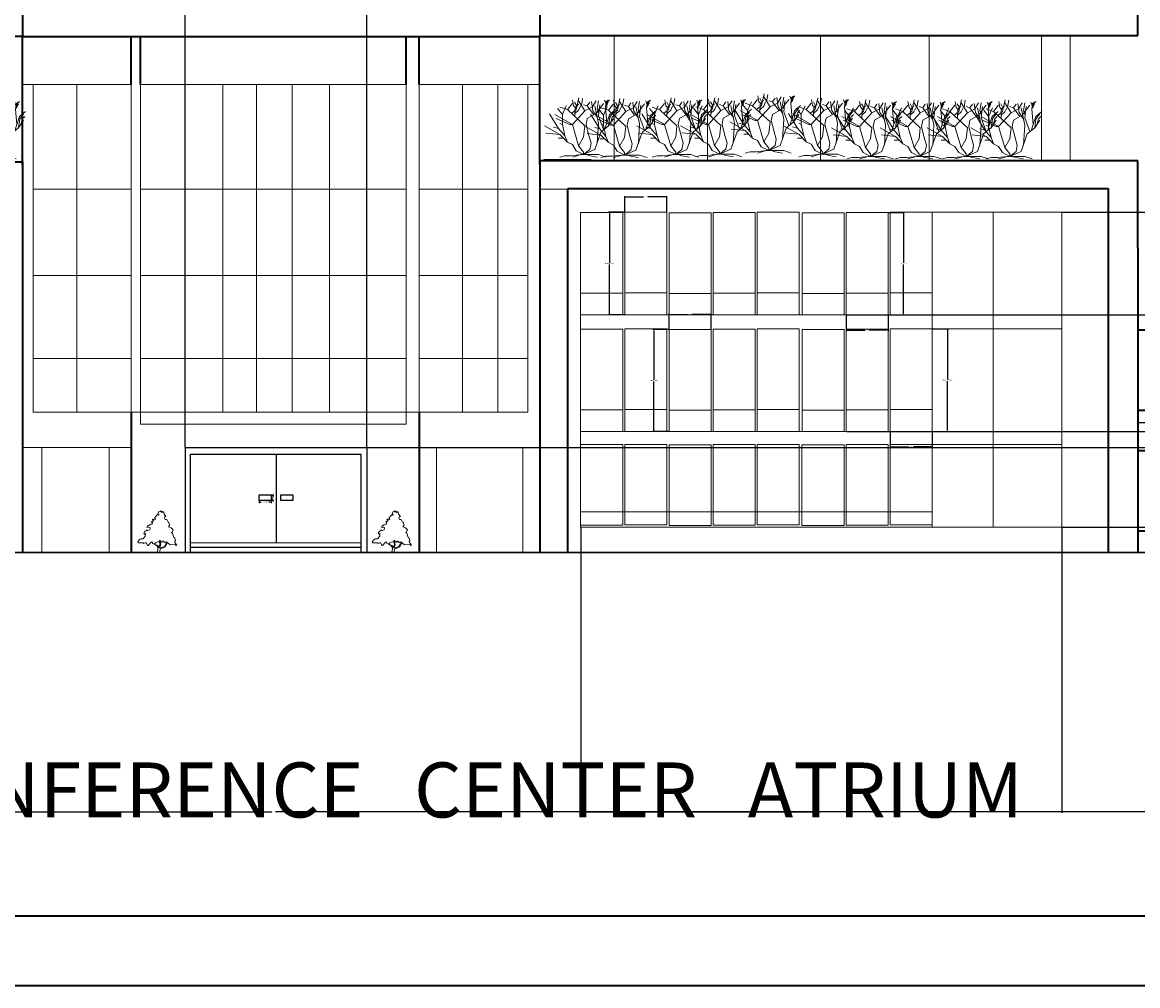
# Model space of a CAD drawing. Units: inches. Extents: x -279 to 364, y -385 to 335.
# Tile 2 of 9: x 7 to 238, y -385 to -185. Entities that reach past the tile are written whole.
import ezdxf

# ---------------------------------------------------------------- set-up
doc = ezdxf.new("R2010")
doc.units = ezdxf.units.IN
doc.header["$MEASUREMENT"] = 0
for name, color, linetype, lineweight in [('A-ANNO-DIMS', 2, 'Continuous', 18), ('A-ANNO-TEXT', 7, 'Continuous', 25), ('A-ANNO-TTLB', 7, 'Continuous', 35), ('A-DOOR', 3, 'Continuous', 25), ('A-GLAZ', 4, 'Continuous', 18), ('A-GLAZ-CURT', 4, 'Continuous', 18), ('A-WALL', 7, 'Continuous', 35), ('C-TOPO', 32, 'Continuous', 30), ('L-PLNT', 94, 'Continuous', 13)]:
    doc.layers.add(name, color=color, linetype=linetype, lineweight=lineweight)
doc.styles.get("Standard").update_dxf_attribs({"font": 'arial.ttf'})
doc.dimstyles.get("Standard").update_dxf_attribs({"dimtxt": 0.18, "dimasz": 0.18, "dimexe": 0.18, "dimexo": 0.0625, "dimgap": 0.09, "dimtad": 0, "dimtih": 1, "dimtoh": 1, "dimdec": 4, "dimzin": 0, "dimdsep": 46, "dimtxsty": 'Standard', "dimcen": 0.09, "dimadec": 0, "dimazin": 0, "dimtfac": 1, "dimtdec": 4, "dimtofl": 0, "dimtmove": 0, "dimatfit": 3, "dimfxl": 1, "dimtolj": 1, "dimtzin": 0, "dimarcsym": 0})

# ---------------------------------------------------------------- blocks, each defined once
blk = doc.blocks.new('*U2')
for p, q in [((-12.471, 19.775), (-12.898, 22.044)), ((-11.433, 18.289), (-10.457, 22.749)), ((-8.16, 17.76), (-10.56, 21.6)), ((-9.48, 19.775), (-8.992, 22.592)), ((-5.28, 19.2), (-3.84, 21.6)), ((-3.377, 18.602), (-2.888, 21.575)), ((-0.508, 21.888), (-0.081, 20.558)), ((0.041, 20.714), (1.384, 22.044)), ((0.102, 21.34), (0.835, 21.888)), ((-16.8, 16.32), (-18.72, 18.72)), ((-14.88, 18.24), (-17.76, 19.2)), ((-16.8, 16.32), (-15.36, 19.68)), ((-14.88, 18.24), (-12.96, 20.64)), ((-8.16, 12), (-14.88, 18.24)), ((-13.325, 16.724), (-11.433, 18.289)), ((-12.96, 12.48), (-8.16, 17.76)), ((-11.677, 19.071), (-12.471, 19.775)), ((-11.28, 19.619), (-12.104, 21.184)), ((-12.043, 15.628), (-11.921, 18.836)), ((-11.982, 16.802), (-10.579, 18.054)), ((-11.921, 18.836), (-10.64, 20.401)), ((-10.579, 18.054), (-9.846, 19.697)), ((-7.2, 19.68), (-8.64, 20.16)), ((-8.16, 17.76), (-5.28, 19.2)), ((-7.2, 19.68), (-6.24, 21.12)), ((-4.8, 16.32), (-7.2, 19.68)), ((-5.086, 17.741), (-5.513, 21.34)), ((-3.377, 15.315), (-5.086, 17.819)), ((-2.88, 12.96), (-4.32, 19.68)), ((-3.84, 16.8), (-0.96, 20.64)), ((-2.766, 16.802), (-3.377, 18.602)), ((-2.88, 15.84), (-2.4, 20.16)), ((-0.203, 19.149), (0.102, 21.34)), ((0.346, 13.203), (-0.203, 19.149)), ((-0.142, 19.384), (0.59, 20.401)), ((-0.02, 20.01), (0.896, 21.105)), ((1.323, 16.254), (3.642, 18.289)), ((1.44, 15.36), (2.88, 17.28)), ((-18.24, 11.04), (-21.755, 16.655)), ((-12.96, 12.48), (-19.68, 16.32)), ((-13.92, 12.48), (-19.2, 14.88)), ((-16.8, 12.48), (-17.76, 12.96)), ((-16.8, 12.48), (-16.8, 16.32)), ((-7.68, 12.48), (-7.2, 14.88)), ((-7.2, 14.88), (-3.84, 16.8)), ((-3.36, 5.28), (-2.88, 12.96)), ((-0.96, 10.56), (-2.88, 15.84)), ((-0.48, 10.8), (0.346, 13.203)), ((0.346, 13.203), (1.323, 16.254)), ((0.96, 12), (1.44, 15.36)), ((0.96, 12), (2.88, 14.88)), ((1.92, 13.44), (2.4, 15.36)), ((2.4, 15.36), (3.36, 16.32)), ((-17.76, 8.64), (-23.663, 11.961)), ((-17.76, 8.64), (-23.128, 9.222)), ((-18.24, 11.04), (-20.16, 11.52)), ((-15.84, 8.16), (-18.24, 11.04)), ((-14.88, 5.76), (-17.76, 8.64)), ((-15.84, 8.16), (-16.8, 12.48)), ((-12.96, 12.48), (-13.92, 12.48)), ((-10.56, 4.32), (-12.96, 12.48)), ((-8.64, 7.68), (-8.16, 12)), ((-6.72, 8.64), (-7.68, 12.48)), ((-5.76, 5.28), (-6.72, 8.64)), ((-4.32, 2.88), (-1.92, 9.6)), ((-1.92, 9.6), (0.96, 12)), ((-16.32, 7.2), (-18.24, 7.2)), ((-14.88, 5.76), (-15.84, 8.16)), ((-12.96, 4.8), (-14.88, 5.76)), ((-11.52, 2.4), (-12.96, 4.8)), ((-10.56, 4.32), (-8.64, 7.68)), ((-8.64, 1.92), (-10.56, 4.32)), ((-6.24, 2.88), (-5.76, 5.28)), ((-15.84, 0.48), (-17.76, 0)), ((-13.44, 0.48), (-15.84, 0.48)), ((-9.6, 0.96), (-13.44, 0.48)), ((-9.6, 0.96), (-12.96, 0)), ((-8.64, 0.96), (-11.52, 2.4)), ((-9.6, 0.96), (-7.68, 0.96)), ((-8.64, 0.96), (-4.32, 2.88)), ((-8.64, 0.96), (-6.24, 2.88)), ((-8.64, 0.96), (-8.64, 1.92)), ((-8.64, 0.96), (-2.88, 0.96)), ((-7.68, 0.96), (-6.24, 0.48)), ((-6.24, 0.48), (-3.36, 0)), ((-2.88, 0.96), (0, 0))]:
    blk.add_line(p, q)
blk = doc.blocks.new('*U4')
for points in [[(22.0124, 137.721), (18.5475, 141.5624), (15.5282, 138.2446), (13.8028, 139.3505), (13.3714, 142.1153), (11.2148, 143.2214), (8.1954, 140.4564), (4.7447, 141.0094), (2.1567, 136.0326), (2.1567, 131.6088), (5.6074, 129.9499), (3.0193, 128.2909), (0.4313, 130.5029), (-6.9015, 123.3141), (-6.9015, 121.6552), (-9.9208, 119.9963), (-9.0581, 118.3373), (-6.9015, 115.0195), (-10.7835, 112.2546), (-14.6656, 115.0195), (-16.8222, 114.4665), (-17.6849, 112.2546), (-14.6656, 111.7016), (-14.2342, 107.2778), (-17.6065, 107.8307), (-21.5669, 103.9599), (-17.2536, 103.4069), (-18.9789, 97.8771), (-22.8609, 97.3241), (-27.1743, 94.5593), (-32.3504, 91.7944), (-32.7817, 94.0063), (-36.6638, 85.7116), (-29.7624, 87.3705), (-25.449, 84.6056), (-26.743, 77.9699), (-34.507, 75.205), (-37.9578, 77.4169), (-39.2518, 74.099), (-42.2711, 73.5461), (-44.8592, 70.2282), (-47.8786, 66.3574), (-43.9965, 63.0395), (-41.4085, 64.6985), (-44.3346, 59.8898), (-42.2089, 60.1377), (-42.5159, 55.7849), (-49.6039, 46.4502), (-58.2307, 45.8972), (-62.1127, 43.6853), (-68.5828, 36.4966), (-65.9947, 32.0727), (-50.0352, 32.6257), (-47.0159, 30.4138), (-39.6831, 33.7317), (-34.507, 22.6721), (-32.3504, 22.6721), (-22.4296, 34.8376), (-19.4102, 36.4966), (-17.2536, 33.7317), (-17.2536, 29.8608), (-13.8028, 28.7549), (-9.0581, 28.7549), (-7.3328, 32.6257), (-1.7254, 35.3906), (3.8821, 35.9436), (6.4701, 38.1555), (6.9014, 38.7085), (8.1954, 41.4734), (9.9208, 40.3674), (11.2148, 35.9436), (14.2341, 37.6025), (15.0968, 36.4966), (15.9595, 33.7317), (18.9789, 38.7085), (21.9982, 38.7085), (23.2922, 36.4966), (21.9982, 34.2847), (25.4489, 35.3906), (26.743, 33.7317), (29.7623, 35.9436), (32.7817, 34.8376), (38.8204, 28.7549), (41.4084, 27.6489), (43.5651, 25.437), (61.6813, 27.0959), (65.132, 23.7781), (67.7201, 24.884), (60.8186, 33.7317), (60.3873, 37.0495), (62.544, 40.3674), (58.662, 50.874), (56.5053, 50.874), (52.1919, 66.3574), (47.8785, 66.9103), (50.4665, 69.1222), (53.9172, 77.9699), (47.0158, 85.1586), (38.3891, 87.9235), (42.2711, 94.0063)], [(42.2711, 94.0063), (38.8204, 104.5129), (36.6637, 104.5129), (32.3503, 113.9135), (29.7623, 113.3605), (26.743, 113.3605), (24.5862, 117.7844), (25.8802, 123.8671), (29.331, 123.8671), (22.8609, 131.6088), (21.9982, 137.6916)], [(8.1954, 40.3674), (11.2148, 27.6489), (8.1954, 13.8245), (24.5862, 19.9072), (32.7817, 34.2847)], [(-12.9401, 28.7549), (-2.588, 22.1191), (0.8626, 17.6953), (1.7253, 11.6125), (0, 0)], [(-9.9208, 28.2019), (0, 23.2251), (3.4507, 19.9072), (4.7447, 15.4834), (8.6267, 27.0959), (6.4701, 37.6025)], [(34.5071, 33.1787), (27.1743, 18.2483), (9.0581, 10.5066), (7.7641, 3.8708), (8.1954, 0)]]:
    blk.add_lwpolyline(points)
blk = doc.blocks.new('WIN-SIDE-SINGLE')
for p, q in [((8.72, 16.72), (0, 16.72)), ((0, 16.72), (0, 15.47)), ((8.72, 0), (8.72, 16.72)), ((0, 15.47), (0, 0)), ((0, 0), (8.72, 0))]:
    blk.add_line(p, q)
blk = doc.blocks.new('WIN-ATRIUM-BAND')
for p, q in [((0, 0), (0, 21.21)), ((0, 21.21), (8.71, 21.21)), ((8.71, 21.21), (8.71, 19.97)), ((8.71, 19.97), (8.71, 0)), ((8.71, 4.5), (0, 4.5))]:
    blk.add_line(p, q)
blk = doc.blocks.new('WIN-ATRIUM-BAND-2')
for p, q in [((0, 0), (0, 21.26)), ((0, 21.26), (8.71, 21.26)), ((8.71, 21.26), (8.71, 20.01)), ((8.71, 20.01), (8.71, 0)), ((8.71, 4.54), (0, 4.54))]:
    blk.add_line(p, q)
blk = doc.blocks.new('WIN-ATRIUM-BAND-3')
for p, q in [((0, 0), (0, 21.12)), ((0, 21.12), (8.71, 21.12)), ((8.71, 21.12), (8.71, 19.88)), ((8.71, 19.88), (8.71, 0)), ((8.71, 4.4), (0, 4.4))]:
    blk.add_line(p, q)
blk = doc.blocks.new('PROJECTION-SIDE')
for p, q in [((0, 16.72), (5.49, 16.72)), ((5.49, 16.72), (5.49, 0)), ((5.49, 0), (0, 0))]:
    blk.add_line(p, q)
blk = doc.blocks.new('PULL-ATRIUM')
for p, q in [((0, 1.18), (2.49, 1.18)), ((0, 0), (0, 1.18)), ((2.49, 1.18), (2.49, 0)), ((2.49, 0), (0, 0))]:
    blk.add_line(p, q)
blk = doc.blocks.new('WIN-RIBBON-END')
for p, q in [((0, 0), (0, 21.26)), ((0, 21.26), (8.72, 21.26)), ((8.72, 21.26), (8.72, 20.01)), ((8.72, 20.01), (8.72, 4.54)), ((8.72, 4.54), (0, 4.54))]:
    blk.add_line(p, q)
blk = doc.blocks.new('*D52')
at = {"layer": 'A-ANNO-DIMS', "color": 0, "lineweight": -2, "transparency": 16777216}
for p, q in [((186.63, -224.9), (189.93, -224.9)), ((189.75, -225.08), (189.75, -235.32)), ((189.75, -245.93), (189.75, -235.69)), ((186.63, -246.11), (189.93, -246.11))]:
    blk.add_line(p, q, dxfattribs=at)
at = {"layer": 'A-ANNO-DIMS', "color": 0, "transparency": 16777216}
for points in [[(189.72, -225.08), (189.78, -225.08), (189.75, -224.9)], [(189.72, -245.93), (189.78, -245.93), (189.75, -246.11)]]:
    blk.add_solid(points, dxfattribs=at)
at = {"layer": 'Defpoints', "color": 0, "transparency": 16777216}
for p in [(186.57, -224.9), (189.75, -224.9), (186.57, -246.11)]:
    blk.add_point(p, dxfattribs=at)
at = {"layer": 'A-ANNO-DIMS', "color": 0, "transparency": 16777216, "insert": (189.75, -235.51), "char_height": 0.18, "attachment_point": 5}
blk.add_mtext('\\A1;LIGHT A 21 TYP.', dxfattribs=at)
blk = doc.blocks.new('*D53')
at = {"layer": 'A-ANNO-DIMS', "color": 0, "lineweight": -2, "transparency": 16777216}
for p, q in [((177.85, -246.17), (177.85, -249.47)), ((186.57, -246.17), (186.57, -249.47)), ((178.03, -249.29), (181.75, -249.29)), ((186.39, -249.29), (182.67, -249.29))]:
    blk.add_line(p, q, dxfattribs=at)
at = {"layer": 'A-ANNO-DIMS', "color": 0, "transparency": 16777216}
for points in [[(178.03, -249.26), (178.03, -249.32), (177.85, -249.29)], [(186.39, -249.26), (186.39, -249.32), (186.57, -249.29)]]:
    blk.add_solid(points, dxfattribs=at)
at = {"layer": 'Defpoints', "color": 0, "transparency": 16777216}
for p in [(177.85, -246.11), (186.57, -246.11), (186.57, -249.29)]:
    blk.add_point(p, dxfattribs=at)
at = {"layer": 'A-ANNO-DIMS', "color": 0, "transparency": 16777216, "insert": (182.21, -249.29), "char_height": 0.18, "attachment_point": 5}
blk.add_mtext('\\A1;9 TYP.', dxfattribs=at)
blk = doc.blocks.new('*D54')
at = {"layer": 'A-ANNO-DIMS', "color": 0, "lineweight": -2, "transparency": 16777216}
for p, q in [((131.88, -224.85), (128.57, -224.85)), ((128.75, -225.03), (128.75, -235.3)), ((128.75, -245.93), (128.75, -235.67)), ((131.88, -246.11), (128.57, -246.11))]:
    blk.add_line(p, q, dxfattribs=at)
at = {"layer": 'A-ANNO-DIMS', "color": 0, "transparency": 16777216}
for points in [[(128.72, -225.03), (128.78, -225.03), (128.75, -224.85)], [(128.72, -245.93), (128.78, -245.93), (128.75, -246.11)]]:
    blk.add_solid(points, dxfattribs=at)
at = {"layer": 'Defpoints', "color": 0, "transparency": 16777216}
for p in [(128.75, -224.85), (131.94, -224.85), (131.94, -246.11)]:
    blk.add_point(p, dxfattribs=at)
at = {"layer": 'A-ANNO-DIMS', "color": 0, "transparency": 16777216, "insert": (128.75, -235.48), "char_height": 0.18, "attachment_point": 5}
blk.add_mtext('\\A1;LIGHT B 21 TYP.', dxfattribs=at)
blk = doc.blocks.new('*D55')
at = {"layer": 'A-ANNO-DIMS', "color": 0, "lineweight": -2, "transparency": 16777216}
for p, q in [((131.94, -224.79), (131.94, -221.49)), ((132.12, -221.67), (135.84, -221.67)), ((140.47, -221.67), (136.75, -221.67)), ((140.65, -224.79), (140.65, -221.49))]:
    blk.add_line(p, q, dxfattribs=at)
at = {"layer": 'A-ANNO-DIMS', "color": 0, "transparency": 16777216}
for points in [[(132.12, -221.64), (132.12, -221.7), (131.94, -221.67)], [(140.47, -221.64), (140.47, -221.7), (140.65, -221.67)]]:
    blk.add_solid(points, dxfattribs=at)
at = {"layer": 'Defpoints', "color": 0, "transparency": 16777216}
for p in [(140.65, -221.67), (131.94, -224.85), (140.65, -224.85)]:
    blk.add_point(p, dxfattribs=at)
at = {"layer": 'A-ANNO-DIMS', "color": 0, "transparency": 16777216, "insert": (136.3, -221.67), "char_height": 0.18, "attachment_point": 5}
blk.add_mtext('\\A1;9 TYP.', dxfattribs=at)
blk = doc.blocks.new('*D56')
at = {"layer": 'A-ANNO-DIMS', "color": 0, "lineweight": -2, "transparency": 16777216}
for p, q in [((141.08, -249.18), (137.8, -249.18)), ((137.98, -249.36), (137.98, -259.56)), ((137.98, -270.13), (137.98, -259.93)), ((141.08, -270.31), (137.8, -270.31))]:
    blk.add_line(p, q, dxfattribs=at)
at = {"layer": 'A-ANNO-DIMS', "color": 0, "transparency": 16777216}
for points in [[(137.95, -249.36), (138.01, -249.36), (137.98, -249.18)], [(137.95, -270.13), (138.01, -270.13), (137.98, -270.31)]]:
    blk.add_solid(points, dxfattribs=at)
at = {"layer": 'Defpoints', "color": 0, "transparency": 16777216}
for p in [(137.98, -249.18), (141.15, -249.18), (141.15, -270.31)]:
    blk.add_point(p, dxfattribs=at)
at = {"layer": 'A-ANNO-DIMS', "color": 0, "transparency": 16777216, "insert": (137.98, -259.74), "char_height": 0.18, "attachment_point": 5}
blk.add_mtext('\\A1;LIGHT C 21 TYP.', dxfattribs=at)
blk = doc.blocks.new('*D57')
at = {"layer": 'A-ANNO-DIMS', "color": 0, "lineweight": -2, "transparency": 16777216}
for p, q in [((141.15, -249.12), (141.15, -245.83)), ((141.33, -246.01), (145.05, -246.01)), ((149.68, -246.01), (145.96, -246.01)), ((149.86, -249.12), (149.86, -245.83))]:
    blk.add_line(p, q, dxfattribs=at)
at = {"layer": 'A-ANNO-DIMS', "color": 0, "transparency": 16777216}
for points in [[(141.33, -245.98), (141.33, -246.04), (141.15, -246.01)], [(149.68, -245.98), (149.68, -246.04), (149.86, -246.01)]]:
    blk.add_solid(points, dxfattribs=at)
at = {"layer": 'Defpoints', "color": 0, "transparency": 16777216}
for p in [(149.86, -246.01), (141.15, -249.18), (149.86, -249.18)]:
    blk.add_point(p, dxfattribs=at)
at = {"layer": 'A-ANNO-DIMS', "color": 0, "transparency": 16777216, "insert": (145.5, -246.01), "char_height": 0.18, "attachment_point": 5}
blk.add_mtext('\\A1;9 TYP.', dxfattribs=at)
blk = doc.blocks.new('*D58')
at = {"layer": 'A-ANNO-DIMS', "color": 0, "lineweight": -2, "transparency": 16777216}
for p, q in [((195.77, -249.05), (199.08, -249.05)), ((198.9, -249.23), (198.9, -259.5)), ((198.9, -270.13), (198.9, -259.86)), ((195.77, -270.31), (199.08, -270.31))]:
    blk.add_line(p, q, dxfattribs=at)
at = {"layer": 'A-ANNO-DIMS', "color": 0, "transparency": 16777216}
for points in [[(198.87, -249.23), (198.93, -249.23), (198.9, -249.05)], [(198.87, -270.13), (198.93, -270.13), (198.9, -270.31)]]:
    blk.add_solid(points, dxfattribs=at)
at = {"layer": 'Defpoints', "color": 0, "transparency": 16777216}
for p in [(195.71, -249.05), (198.9, -249.05), (195.71, -270.31)]:
    blk.add_point(p, dxfattribs=at)
at = {"layer": 'A-ANNO-DIMS', "color": 0, "transparency": 16777216, "insert": (198.9, -259.68), "char_height": 0.18, "attachment_point": 5}
blk.add_mtext('\\A1;END PANEL 21 TYP.', dxfattribs=at)
blk = doc.blocks.new('*D59')
at = {"layer": 'A-ANNO-DIMS', "color": 0, "lineweight": -2, "transparency": 16777216}
for p, q in [((186.99, -270.37), (186.99, -273.67)), ((195.71, -270.37), (195.71, -273.67)), ((187.17, -273.49), (190.89, -273.49)), ((195.53, -273.49), (191.81, -273.49))]:
    blk.add_line(p, q, dxfattribs=at)
at = {"layer": 'A-ANNO-DIMS', "color": 0, "transparency": 16777216}
for points in [[(187.17, -273.46), (187.17, -273.52), (186.99, -273.49)], [(195.53, -273.46), (195.53, -273.52), (195.71, -273.49)]]:
    blk.add_solid(points, dxfattribs=at)
at = {"layer": 'Defpoints', "color": 0, "transparency": 16777216}
for p in [(186.99, -270.31), (195.71, -270.31), (195.71, -273.49)]:
    blk.add_point(p, dxfattribs=at)
at = {"layer": 'A-ANNO-DIMS', "color": 0, "transparency": 16777216, "insert": (191.35, -273.49), "char_height": 0.18, "attachment_point": 5}
blk.add_mtext('\\A1;9 TYP.', dxfattribs=at)
blk = doc.blocks.new('*D69')
at = {"layer": 'A-ANNO-DIMS', "color": 0, "lineweight": -2, "transparency": 16777216}
for p, q in [((238.34, -265.99), (238.34, -268.61)), ((243.83, -265.99), (243.83, -268.61)), ((238.52, -268.43), (240.62, -268.43)), ((243.65, -268.43), (241.54, -268.43))]:
    blk.add_line(p, q, dxfattribs=at)
at = {"layer": 'A-ANNO-DIMS', "color": 0, "transparency": 16777216}
for points in [[(238.52, -268.4), (238.52, -268.46), (238.34, -268.43)], [(243.65, -268.4), (243.65, -268.46), (243.83, -268.43)]]:
    blk.add_solid(points, dxfattribs=at)
at = {"layer": 'Defpoints', "color": 0, "transparency": 16777216}
for p in [(238.34, -265.92), (243.83, -265.92), (243.83, -268.43)]:
    blk.add_point(p, dxfattribs=at)
at = {"layer": 'A-ANNO-DIMS', "color": 0, "transparency": 16777216, "insert": (241.08, -268.43), "char_height": 0.18, "attachment_point": 5}
blk.add_mtext('\\A1;5 TYP.', dxfattribs=at)
blk = doc.blocks.new('*D70')
at = {"layer": 'A-ANNO-DIMS', "color": 0, "lineweight": -2, "transparency": 16777216}
for p, q in [((56.09, -284.66), (56.09, -285.15)), ((56.27, -284.97), (56.53, -284.97)), ((58.4, -284.97), (58.14, -284.97)), ((58.58, -284.66), (58.58, -285.15))]:
    blk.add_line(p, q, dxfattribs=at)
at = {"layer": 'A-ANNO-DIMS', "color": 0, "transparency": 16777216}
for points in [[(56.27, -284.94), (56.27, -285), (56.09, -284.97)], [(58.4, -284.94), (58.4, -285), (58.58, -284.97)]]:
    blk.add_solid(points, dxfattribs=at)
at = {"layer": 'Defpoints', "color": 0, "transparency": 16777216}
for p in [(56.09, -284.6), (58.58, -284.6), (58.58, -284.97)]:
    blk.add_point(p, dxfattribs=at)
at = {"layer": 'A-ANNO-DIMS', "color": 0, "transparency": 16777216, "insert": (57.33, -284.97), "char_height": 0.18, "attachment_point": 5}
blk.add_mtext('\\A1;PULL 2 TYP.', dxfattribs=at)
blk = doc.blocks.new('*D71')
at = {"layer": 'A-ANNO-DIMS', "color": 0, "lineweight": -2, "transparency": 16777216}
for p, q in [((58.64, -283.42), (59.13, -283.42)), ((58.95, -283.6), (58.95, -283.83)), ((58.95, -284.42), (58.95, -284.19)), ((58.64, -284.6), (59.13, -284.6))]:
    blk.add_line(p, q, dxfattribs=at)
at = {"layer": 'A-ANNO-DIMS', "color": 0, "transparency": 16777216}
for points in [[(58.92, -283.6), (58.98, -283.6), (58.95, -283.42)], [(58.92, -284.42), (58.98, -284.42), (58.95, -284.6)]]:
    blk.add_solid(points, dxfattribs=at)
at = {"layer": 'Defpoints', "color": 0, "transparency": 16777216}
for p in [(58.58, -283.42), (58.95, -283.42), (58.58, -284.6)]:
    blk.add_point(p, dxfattribs=at)
at = {"layer": 'A-ANNO-DIMS', "color": 0, "transparency": 16777216, "insert": (58.95, -284.01), "char_height": 0.18, "attachment_point": 5}
blk.add_mtext('\\A1;1 TYP.', dxfattribs=at)
blk = doc.blocks.new('*D97')
at = {"layer": 'A-ANNO-DIMS', "color": 0, "lineweight": -2, "transparency": 16777216}
for p, q in [((243.83, -291), (243.83, -349.37)), ((-125.57, -295.46), (-125.57, -349.37)), ((-125.39, -349.19), (58.74, -349.19)), ((243.65, -349.19), (59.52, -349.19))]:
    blk.add_line(p, q, dxfattribs=at)
at = {"layer": 'A-ANNO-DIMS', "color": 0, "transparency": 16777216}
for points in [[(-125.39, -349.16), (-125.39, -349.22), (-125.57, -349.19)], [(243.65, -349.16), (243.65, -349.22), (243.83, -349.19)]]:
    blk.add_solid(points, dxfattribs=at)
at = {"layer": 'Defpoints', "color": 0, "transparency": 16777216}
for p in [(243.83, -290.94), (-125.57, -295.4), (243.83, -349.19)]:
    blk.add_point(p, dxfattribs=at)
at = {"layer": 'A-ANNO-DIMS', "color": 0, "transparency": 16777216, "insert": (59.13, -349.19), "char_height": 0.18, "attachment_point": 5}
blk.add_mtext('\\A1;369.4', dxfattribs=at)
blk = doc.blocks.new('*D112')
at = {"layer": 'A-ANNO-DIMS', "color": 0, "lineweight": -2, "transparency": 16777216}
for p, q in [((177.91, -246.11), (361.74, -246.11)), ((361.56, -246.29), (361.56, -258.03)), ((361.56, -270.13), (361.56, -258.39)), ((177.91, -270.31), (361.74, -270.31))]:
    blk.add_line(p, q, dxfattribs=at)
at = {"layer": 'A-ANNO-DIMS', "color": 0, "transparency": 16777216}
for points in [[(361.53, -246.29), (361.59, -246.29), (361.56, -246.11)], [(361.53, -270.13), (361.59, -270.13), (361.56, -270.31)]]:
    blk.add_solid(points, dxfattribs=at)
at = {"layer": 'Defpoints', "color": 0, "transparency": 16777216}
for p in [(177.85, -246.11), (177.85, -270.31), (361.56, -270.31)]:
    blk.add_point(p, dxfattribs=at)
at = {"layer": 'A-ANNO-DIMS', "color": 0, "transparency": 16777216, "insert": (361.56, -258.21), "char_height": 0.18, "attachment_point": 5}
blk.add_mtext('\\A1;24.193', dxfattribs=at)
blk = doc.blocks.new('*D113')
at = {"layer": 'A-ANNO-DIMS', "color": 0, "lineweight": -2, "transparency": 16777216}
for p, q in [((122.8, -290.21), (122.8, -349.37)), ((222.59, -290.21), (222.59, -349.37)), ((122.98, -349.19), (172.37, -349.19)), ((222.41, -349.19), (173.02, -349.19))]:
    blk.add_line(p, q, dxfattribs=at)
at = {"layer": 'A-ANNO-DIMS', "color": 0, "transparency": 16777216}
for points in [[(122.98, -349.16), (122.98, -349.22), (122.8, -349.19)], [(222.41, -349.16), (222.41, -349.22), (222.59, -349.19)]]:
    blk.add_solid(points, dxfattribs=at)
at = {"layer": 'Defpoints', "color": 0, "transparency": 16777216}
for p in [(122.8, -290.14), (222.59, -290.14), (222.59, -349.19)]:
    blk.add_point(p, dxfattribs=at)
at = {"layer": 'A-ANNO-DIMS', "color": 0, "transparency": 16777216, "insert": (172.7, -349.19), "char_height": 0.18, "attachment_point": 5}
blk.add_mtext('\\A1;99.8', dxfattribs=at)
blk = doc.blocks.new('*D114')
at = {"layer": 'A-ANNO-DIMS', "color": 0, "lineweight": -2, "transparency": 16777216}
for p, q in [((222.66, -224.85), (361.74, -224.85)), ((361.56, -225.03), (361.56, -257.32)), ((361.56, -289.96), (361.56, -257.68)), ((222.66, -290.14), (361.74, -290.14))]:
    blk.add_line(p, q, dxfattribs=at)
at = {"layer": 'A-ANNO-DIMS', "color": 0, "transparency": 16777216}
for points in [[(361.53, -225.03), (361.59, -225.03), (361.56, -224.85)], [(361.53, -289.96), (361.59, -289.96), (361.56, -290.14)]]:
    blk.add_solid(points, dxfattribs=at)
at = {"layer": 'Defpoints', "color": 0, "transparency": 16777216}
for p in [(222.59, -224.85), (361.56, -224.85), (222.59, -290.14)]:
    blk.add_point(p, dxfattribs=at)
at = {"layer": 'A-ANNO-DIMS', "color": 0, "transparency": 16777216, "insert": (361.56, -257.5), "char_height": 0.18, "attachment_point": 5}
blk.add_mtext('\\A1;65.29', dxfattribs=at)
blk = doc.blocks.new('*D115')
at = {"layer": 'A-ANNO-DIMS', "color": 0, "lineweight": -2, "transparency": 16777216}
for p, q in [((40.79, -273.55), (40.79, -77.65)), ((40.97, -77.83), (59.16, -77.83)), ((78.28, -77.83), (60.09, -77.83)), ((78.46, -273.55), (78.46, -77.65))]:
    blk.add_line(p, q, dxfattribs=at)
at = {"layer": 'A-ANNO-DIMS', "color": 0, "transparency": 16777216}
for points in [[(40.97, -77.8), (40.97, -77.86), (40.79, -77.83)], [(78.28, -77.8), (78.28, -77.86), (78.46, -77.83)]]:
    blk.add_solid(points, dxfattribs=at)
at = {"layer": 'Defpoints', "color": 0, "transparency": 16777216}
for p in [(78.46, -77.83), (40.79, -273.62), (78.46, -273.62)]:
    blk.add_point(p, dxfattribs=at)
at = {"layer": 'A-ANNO-DIMS', "color": 0, "transparency": 16777216, "insert": (59.62, -77.83), "char_height": 0.18, "attachment_point": 5}
blk.add_mtext('\\A1;37.665', dxfattribs=at)
blk = doc.blocks.new('*D116')
at = {"layer": 'A-ANNO-DIMS', "color": 0, "lineweight": -2, "transparency": 16777216}
for p, q in [((78.52, -273.62), (361.74, -273.62)), ((361.56, -273.8), (361.56, -284.32)), ((361.56, -295.22), (361.56, -284.69)), ((78.52, -295.4), (361.74, -295.4))]:
    blk.add_line(p, q, dxfattribs=at)
at = {"layer": 'A-ANNO-DIMS', "color": 0, "transparency": 16777216}
for points in [[(361.53, -273.8), (361.59, -273.8), (361.56, -273.62)], [(361.53, -295.22), (361.59, -295.22), (361.56, -295.4)]]:
    blk.add_solid(points, dxfattribs=at)
at = {"layer": 'Defpoints', "color": 0, "transparency": 16777216}
for p in [(78.46, -273.62), (361.56, -273.62), (78.46, -295.4)]:
    blk.add_point(p, dxfattribs=at)
at = {"layer": 'A-ANNO-DIMS', "color": 0, "transparency": 16777216, "insert": (361.56, -284.51), "char_height": 0.18, "attachment_point": 5}
blk.add_mtext('\\A1;21.78', dxfattribs=at)

msp = doc.modelspace()

# ---------------------------------------------------------------- linework, layer by layer
at = {"layer": 'A-ANNO-TTLB'}
for points in [[(-279.2289, 334.6468), (364.0508, 334.6468), (364.0508, -385.2219), (-279.2289, -385.2219)], [(-267.2403, 317.5778), (348.1051, 317.5778), (348.1051, -370.8321), (-267.2403, -370.8321)]]:
    msp.add_lwpolyline(points, close=True, dxfattribs=at)
at = {"layer": 'A-DOOR'}
for p, q in [((40.7926, -273.6155), (40.7926, -295.3951)), ((40.7926, -273.6155), (78.4572, -273.6155)), ((41.8827, -295.3951), (41.8827, -275.0371)), ((41.8827, -275.0371), (76.4698, -275.0371)), ((59.633, -275.0371), (59.633, -293.3714)), ((76.4698, -275.0371), (77.2147, -275.0371)), ((77.2147, -275.0371), (77.2147, -295.3951)), ((78.4572, -273.6155), (78.4572, -295.3951)), ((41.8827, -293.3925), (77.2147, -293.3505)), ((41.8827, -294.3193), (77.2147, -294.3193))]:
    msp.add_line(p, q, dxfattribs=at)
at = {"layer": 'A-GLAZ-CURT'}
for p, q in [((129.7541, -188.2171), (129.7541, -214.2107)), ((149.1145, -188.2171), (149.1145, -214.2107)), ((172.5204, -188.2171), (172.5204, -214.2107)), ((195.0593, -188.2171), (195.0593, -214.2107)), ((218.3669, -188.2171), (218.3669, -214.2107)), ((224.3504, -188.2171), (224.3504, -214.2107)), ((7.0091, -198.3492), (29.5321, -198.3492)), ((9.2692, -198.3492), (9.2692, -266.2836)), ((18.2716, -198.3492), (18.2716, -266.2836)), ((29.5321, -198.3492), (29.5321, -266.2836)), ((31.4736, -198.3492), (31.4736, -266.2836)), ((31.4736, -198.3492), (86.6113, -198.3492)), ((40.7926, -198.3492), (40.7926, -266.2836)), ((48.5585, -198.3492), (48.5585, -266.2836)), ((55.5478, -198.3492), (55.5478, -266.2836)), ((62.9254, -198.3492), (62.9254, -266.2836)), ((70.6913, -198.3492), (70.6913, -266.2836)), ((78.4572, -198.3492), (78.4572, -266.2836)), ((86.6113, -198.3492), (86.6113, -266.2836)), ((89.3294, -198.3492), (89.3294, -266.2836)), ((89.3294, -198.3492), (114.3455, -198.3492)), ((98.2602, -198.3492), (98.2602, -266.2836)), ((105.6378, -198.3492), (105.6378, -266.2836)), ((111.8227, -198.3492), (111.8227, -266.2836)), ((9.2692, -220.0327), (29.5321, -220.0327)), ((31.4736, -220.0327), (86.6113, -220.0327)), ((89.3294, -220.0327), (111.8227, -220.0327)), ((114.3455, -220.0327), (120.1078, -220.0327)), ((122.7982, -241.6164), (122.7982, -224.8982)), ((122.7982, -224.8982), (131.5131, -224.8982)), ((131.5131, -224.8982), (131.5131, -226.1417)), ((131.5131, -226.1417), (131.5131, -246.1124)), ((195.7072, -224.8549), (222.5949, -224.8549)), ((195.7072, -290.1425), (195.7072, -226.0984)), ((208.3594, -224.8549), (208.3594, -290.1425)), ((222.5949, -224.8549), (222.5949, -290.1425)), ((9.2692, -237.9317), (29.5321, -237.9317)), ((31.4736, -237.9317), (86.6113, -237.9317)), ((89.3294, -237.9317), (111.8227, -237.9317)), ((131.5131, -241.6164), (122.7982, -241.6164)), ((122.7982, -241.6164), (122.7982, -246.1124)), ((122.7982, -246.1124), (195.7072, -246.1124)), ((122.7982, -246.1124), (122.7982, -273.0151)), ((122.7982, -265.8094), (122.7982, -249.0912)), ((122.7982, -249.0912), (131.5131, -249.0912)), ((131.5131, -249.0912), (131.5131, -250.3347)), ((195.7072, -249.0479), (222.5949, -249.0479)), ((131.5131, -250.3347), (131.5131, -270.3054)), ((9.2692, -255.1934), (29.5321, -255.1934)), ((31.4736, -255.1934), (86.6113, -255.1934)), ((89.3294, -255.1934), (111.8227, -255.1934)), ((131.5131, -265.8094), (122.7982, -265.8094)), ((122.7982, -265.8094), (122.7982, -270.3054)), ((9.2692, -266.2836), (111.8227, -266.2836)), ((31.4736, -266.2836), (31.4736, -268.7642)), ((86.6113, -268.7642), (86.6113, -266.2836)), ((31.4736, -268.7642), (86.6113, -268.7642)), ((122.7982, -270.3054), (195.7072, -270.3054)), ((186.9923, -289.69), (186.9923, -272.9718)), ((186.9923, -272.9718), (195.7072, -272.9718)), ((195.7072, -272.9718), (195.7072, -274.2153)), ((195.7072, -272.9718), (222.5949, -272.9718)), ((7.0091, -273.6155), (29.5321, -273.6155)), ((11.0334, -273.6155), (11.0334, -295.3951)), ((24.9761, -273.6155), (24.9761, -295.3951)), ((89.3294, -273.6155), (114.3455, -273.6155)), ((92.88, -273.6155), (92.88, -295.3951)), ((110.7825, -273.6155), (110.7825, -295.3951)), ((122.7982, -289.7333), (122.7982, -273.0151)), ((122.7982, -273.0151), (131.5131, -273.0151)), ((131.5131, -273.0151), (131.5131, -274.2586)), ((131.5131, -274.2586), (131.5131, -289.7333)), ((195.7072, -274.2153), (195.7072, -289.69)), ((122.7982, -286.9445), (195.7072, -286.9445)), ((131.5131, -289.7333), (122.7982, -289.7333)), ((122.7982, -290.1425), (122.7982, -289.7333)), ((195.7072, -290.1425), (122.7982, -290.1425)), ((195.7072, -289.69), (186.9923, -289.69)), ((222.5949, -290.1425), (195.7072, -290.1425))]:
    msp.add_line(p, q, dxfattribs=at)
at = {"layer": 'A-WALL'}
for p, q in [((7.0091, -130.861), (7.0091, -188.3649)), ((114.3455, -130.7132), (114.3455, -188.2171)), ((238.3359, -188.2171), (238.3359, -130.7132)), ((7.0091, -188.3649), (-116.9812, -188.3649)), ((7.0091, -215.056), (7.0091, -188.3649)), ((7.0091, -188.3649), (114.3455, -188.3649)), ((29.5321, -198.3492), (29.5321, -188.3649)), ((31.4736, -198.3492), (31.4736, -188.3649)), ((86.6113, -198.3492), (86.6113, -188.3649)), ((89.3294, -198.3492), (89.3294, -188.3649)), ((114.3455, -214.9082), (114.3455, -188.2171)), ((114.3455, -188.2171), (238.3359, -188.2171)), ((-116.9812, -214.3585), (7.0091, -214.3585)), ((7.0091, -214.3585), (7.0091, -295.3951)), ((238.3359, -214.2107), (114.3455, -214.2107)), ((114.3455, -214.2107), (114.3455, -295.2473)), ((124.9588, -214.0225), (115.1295, -214.0225)), ((238.3359, -232.2741), (238.3359, -214.2107)), ((120.1078, -295.2473), (120.1078, -219.8849)), ((120.1078, -219.8849), (232.188, -219.8849)), ((232.188, -219.8849), (232.188, -295.2473)), ((238.3359, -232.2741), (238.3359, -295.2473)), ((29.5321, -266.2836), (29.5321, -295.3951)), ((89.3294, -266.2836), (89.3294, -295.3951))]:
    msp.add_line(p, q, dxfattribs=at)
at = {"layer": 'C-TOPO'}
for p, q in [((-116.9812, -295.3951), (195.2296, -295.3951)), ((195.2296, -295.3951), (256.846, -295.3951))]:
    msp.add_line(p, q, dxfattribs=at)

# ---------------------------------------------------------------- block references
at = {"layer": 'A-DOOR'}
for p in [(56.087, -284.596), (60.5938, -284.596)]:
    msp.add_blockref('PULL-ATRIUM', p, dxfattribs=at)
at = {"layer": 'A-GLAZ', "extrusion": (0, 0, -1), "zscale": -1}
for p in [(-140.654, -289.6901), (-168.1439, -289.6901), (-149.8624, -289.8242), (-159.0033, -289.7334), (-177.4259, -289.8242), (-186.5668, -289.7334)]:
    msp.add_blockref('WIN-SIDE-SINGLE', p, dxfattribs=at)
at = {"layer": 'A-GLAZ-CURT'}
for name, p in [('WIN-ATRIUM-BAND-2', (131.939, -246.112)), ('WIN-ATRIUM-BAND-3', (141.1475, -246.112)), ('WIN-ATRIUM-BAND', (150.2885, -246.112)), ('WIN-ATRIUM-BAND-2', (159.429, -246.112)), ('WIN-ATRIUM-BAND-3', (168.711, -246.112)), ('WIN-ATRIUM-BAND', (177.852, -246.112)), ('WIN-RIBBON-END', (186.992, -246.112)), ('WIN-ATRIUM-BAND-2', (131.939, -270.305)), ('WIN-ATRIUM-BAND-3', (141.1475, -270.305)), ('WIN-ATRIUM-BAND', (150.2885, -270.305)), ('WIN-ATRIUM-BAND-2', (159.429, -270.305)), ('WIN-ATRIUM-BAND-3', (168.711, -270.305)), ('WIN-ATRIUM-BAND', (177.852, -270.305)), ('WIN-RIBBON-END', (186.992, -270.305))]:
    msp.add_blockref(name, p, dxfattribs=at)
at = {"layer": 'A-WALL'}
for p in [(238.336, -265.924), (238.336, -290.941)]:
    msp.add_blockref('PROJECTION-SIDE', p, dxfattribs=at)
at = {"layer": 'L-PLNT'}
for name, p, xscale, yscale, zscale in [('*U2', (128.0468, -213.3861), 0.5382827397491715, 0.5382827397491715, 0.5382827397491715), ('*U2', (136.5721, -213.4968), 0.5382827397491715, 0.5382827397491715, 0.5382827397491715), ('*U2', (147.1655, -213.3861), 0.5382827397491715, 0.5382827397491715, 0.5382827397491715), ('*U2', (156.2608, -213.3354), 0.5382827397491715, 0.5382827397491715, 0.5382827397491715), ('*U2', (166.4699, -212.5602), 0.5382827397491715, 0.5382827397491715, 0.5382827397491715), ('*U2', (177.607, -213.3354), 0.5382827397491715, 0.5382827397491715, 0.5382827397491715), ('*U2', (5.6916, -213.7667), 0.5382827397491715, 0.5382827397491715, 0.5382827397491715), ('*U2', (187.5959, -213.7667), 0.5382827397491715, 0.5382827397491715, 0.5382827397491715), ('*U2', (197.6272, -213.7667), 0.5382827397491715, 0.5382827397491715, 0.5382827397491715), ('*U2', (207.4138, -213.7667), 0.5382827397491715, 0.5382827397491715, 0.5382827397491715), ('*U2', (216.4664, -213.7667), 0.5382827397491715, 0.5382827397491715, 0.5382827397491715), ('*U4', (35.0251, -295.3324), 0.0596993606735785, 0.0596993606735785, 0.0596993606735785), ('*U4', (83.6498, -295.3324), 0.0596993606735785, 0.0596993606735785, 0.0596993606735785)]:
    msp.add_blockref(name, p, dxfattribs=dict(at, xscale=xscale, yscale=yscale, zscale=zscale))

# ---------------------------------------------------------------- texts
at = {"layer": 'A-ANNO-TEXT'}
msp.add_text('SIDE   ELEVATION  CONFERENCE   CENTER   ATRIUM', height=11.412549, dxfattribs=at).set_placement((-155.2227, -350.3444))

# ---------------------------------------------------------------- dimensions: what is measured, and where the dimension line sits
at = {"layer": 'A-ANNO-DIMS'}
for base, p1, p2, override, picture, middle in [((78.4572, -77.8255), (40.7926, -273.6155), (78.4572, -273.6155), {"dimdec": 3, "dimlfac": 1, "dimrnd": 0, "dimzin": 0, "dimdsep": 46, "dimlunit": 2}, '*D115', (59.6249, -77.8255)), ((243.8297, -349.1915), (-125.5669, -295.3951), (243.8297, -290.9407), {"dimdec": 1, "dimlfac": 1, "dimrnd": 0, "dimzin": 0, "dimdsep": 46, "dimlunit": 2}, '*D97', (59.1314, -349.1915)), ((222.5949, -349.1915), (122.7982, -290.1425), (222.5949, -290.1425), {"dimdec": 1, "dimlfac": 1, "dimrnd": 0, "dimzin": 0, "dimdsep": 46, "dimlunit": 2}, '*D113', (172.6965, -349.1915))]:
    dim = msp.add_linear_dim(base=base, p1=p1, p2=p2, dimstyle='Standard', override=override, dxfattribs=at)
    dim.commit()
    dim.dimension.update_dxf_attribs({"geometry": picture, "text_midpoint": middle})
for base, p1, p2, text, picture, middle in [((140.6537, -221.6663), (131.9388, -224.8549), (140.6537, -224.8549), '<> TYP.', '*D55', (136.2963, -221.6663)), ((149.8621, -246.0136), (141.1472, -249.1821), (149.8621, -249.1821), '<> TYP.', '*D57', (145.5047, -246.0136)), ((186.5666, -249.2946), (177.8517, -246.1124), (186.5666, -246.1124), '<> TYP.', '*D53', (182.2091, -249.2946)), ((243.8297, -268.4314), (238.3359, -265.9237), (243.8297, -265.9237), '<> TYP.', '*D69', (241.0828, -268.4314)), ((195.7072, -273.494), (186.9923, -270.3054), (195.7072, -270.3054), '<> TYP.', '*D59', (191.3497, -273.494)), ((58.5806, -284.9705), (56.0865, -284.5964), (58.5806, -284.5964), 'PULL <> TYP.', '*D70', (57.3336, -284.9705))]:
    dim = msp.add_linear_dim(base=base, p1=p1, p2=p2, text=text, dimstyle='Standard', override={"dimdec": 0, "dimlfac": 1, "dimrnd": 0, "dimzin": 0, "dimdsep": 46, "dimlunit": 2}, dxfattribs=at)
    dim.commit()
    dim.dimension.update_dxf_attribs({"geometry": picture, "text_midpoint": middle})
for base, p1, p2, text, picture, middle in [((128.7502, -224.8549), (131.9388, -246.1124), (131.9388, -224.8549), 'LIGHT B <> TYP.', '*D54', (128.7502, -235.4837)), ((189.7487, -224.8982), (186.5666, -246.1124), (186.5666, -224.8982), 'LIGHT A <> TYP.', '*D52', (189.7487, -235.5053)), ((137.9787, -249.1821), (141.1472, -270.3054), (141.1472, -249.1821), 'LIGHT C <> TYP.', '*D56', (137.9787, -259.7437)), ((198.8958, -249.0479), (195.7072, -270.3054), (195.7072, -249.0479), 'END PANEL <> TYP.', '*D58', (198.8958, -259.6767)), ((58.9547, -283.4164), (58.5806, -284.5964), (58.5806, -283.4164), '<> TYP.', '*D71', (58.9547, -284.0064))]:
    dim = msp.add_linear_dim(base=base, p1=p1, p2=p2, angle=90, text=text, dimstyle='Standard', override={"dimdec": 0, "dimlfac": 1, "dimrnd": 0, "dimzin": 0, "dimdsep": 46, "dimlunit": 2}, dxfattribs=at)
    dim.commit()
    dim.dimension.update_dxf_attribs({"geometry": picture, "text_midpoint": middle})
for base, p1, p2, override, picture, middle in [((361.5588, -224.8549), (222.5949, -290.1425), (222.5949, -224.8549), {"dimdec": 2, "dimlfac": 1, "dimrnd": 0, "dimzin": 0, "dimdsep": 46, "dimlunit": 2}, '*D114', (361.5588, -257.4987)), ((361.5588, -270.3054), (177.8517, -246.1124), (177.8517, -270.3054), {"dimdec": 3, "dimlfac": 1, "dimrnd": 0, "dimzin": 0, "dimdsep": 46, "dimlunit": 2}, '*D112', (361.5588, -258.2089)), ((361.5588, -273.6155), (78.4572, -295.3951), (78.4572, -273.6155), {"dimdec": 2, "dimlfac": 1, "dimrnd": 0, "dimzin": 0, "dimdsep": 46, "dimlunit": 2}, '*D116', (361.5588, -284.5053))]:
    dim = msp.add_linear_dim(base=base, p1=p1, p2=p2, angle=90, dimstyle='Standard', override=override, dxfattribs=at)
    dim.commit()
    dim.dimension.update_dxf_attribs({"geometry": picture, "text_midpoint": middle})

doc.saveas('drawing.dxf')
